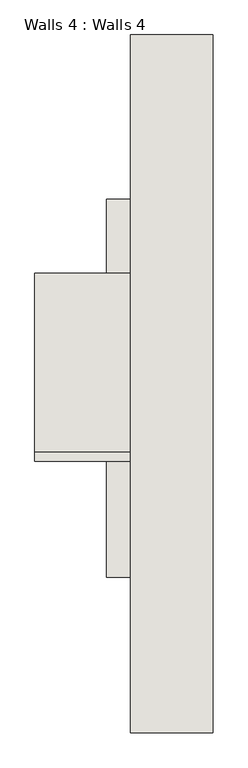
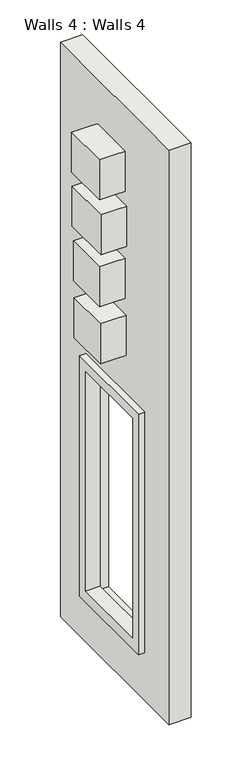
"""IFC4 building model written with IfcOpenShell, lengths in millimetres: wall geometry, Walls 4 : Walls 4."""

from ifc_helpers import new_model, si_unit, frame, origin, place, context, project, spatial, polyline, outline, extrude, source, transform, mapped, element, save


def walls_4_walls_4_b785277b(model_context):
    return source(origin(), model_context, "Body", "SweptSolid", [
        extrude(outline(polyline([(6427.4159582, 6704.0510511), (7343.1184239, 6704.0510511), (7343.1184239, 4418.0510511), (6427.4159582, 4418.0510511), (6427.4159582, 6704.0510511)]), holes=[polyline([(6521.2652695, 6605.6899595), (6521.2652695, 4522.8899595), (7251.0434239, 4522.8899595), (7251.0434239, 6605.6899595), (6521.2652695, 6605.6899595)])]), frame((-12584.6161086, 0.0, 0.0), z_axis=(1.0, 0.0, 0.0), x_axis=(0.0, 1.0, 0.0)), (0.0, 0.0, 1.0), 130.7077729),
        extrude(outline(polyline([(-12758.7083357, 6731.4650508), (-12758.7083357, 7163.2483652), (-12390.4083357, 7163.2483652), (-12390.4083357, 6731.4650508), (-12758.7083357, 6731.4650508)])), frame((0.0, 0.0, 8615.3806189), z_axis=(0.0, 0.0, 1.0), x_axis=(1.0, 0.0, 0.0)), (0.0, 0.0, 1.0), 381.0),
        extrude(outline(polyline([(-12758.7083357, 6708.0602057), (-12758.7083357, 7156.2054395), (-12390.4083357, 7156.2054395), (-12390.4083357, 6708.0602057), (-12758.7083357, 6708.0602057)])), frame((0.0, 0.0, 8107.3806189), z_axis=(0.0, 0.0, 1.0), x_axis=(1.0, 0.0, 0.0)), (0.0, 0.0, 1.0), 381.0),
        extrude(outline(polyline([(-12758.7083357, 6730.7746365), (-12758.7083357, 7137.037243), (-12390.4083357, 7137.037243), (-12390.4083357, 6730.7746365), (-12758.7083357, 6730.7746365)])), frame((0.0, 0.0, 7599.3806189), z_axis=(0.0, 0.0, 1.0), x_axis=(1.0, 0.0, 0.0)), (0.0, 0.0, 1.0), 381.0),
        extrude(outline(polyline([(-12758.7083357, 6716.4341079), (-12758.7083357, 7126.5003631), (-12390.4083357, 7126.5003631), (-12390.4083357, 6716.4341079), (-12758.7083357, 6716.4341079)])), frame((0.0, 0.0, 7065.9806189), z_axis=(0.0, 0.0, 1.0), x_axis=(1.0, 0.0, 0.0)), (0.0, 0.0, 1.0), 381.0),
        extrude(outline(polyline([(6050.8287391, 9420.9325813), (7739.873901, 9420.9325813), (7739.873901, 3962.4), (6050.8287391, 3962.4), (6050.8287391, 9420.9325813)]), holes=[polyline([(6427.4159582, 6704.0510511), (6427.4159582, 4418.0510511), (7341.8159582, 4418.0510511), (7341.8159582, 6704.0510511), (6427.4159582, 6704.0510511)])]), frame((-12527.0272545, 0.0, 0.0), z_axis=(1.0, 0.0, 0.0), x_axis=(0.0, 1.0, 0.0)), (0.0, 0.0, 1.0), 200.1189188),
    ])


if __name__ == "__main__":
    model = new_model("IFC4")
    model_context = context("Model", 3, world=origin())
    ifc_project = project(units=[si_unit("LENGTHUNIT", "METRE", prefix="MILLI")], contexts=[model_context])
    site = spatial("IfcSite", under=ifc_project)
    building = spatial("IfcBuilding", under=site)
    placement = place(None, origin())
    walls_4_walls_4_shape = walls_4_walls_4_b785277b(model_context)
    element("IfcWall", 1, ObjectType="Walls 4 : Walls 4", at=placement, inside=building, context=model_context, shape_type="MappedRepresentation", body=[
        mapped(walls_4_walls_4_shape, transform((0.0, 0.0, 0.0), x_axis=(1.0, 0.0, 0.0), y_axis=(0.0, 1.0, 0.0), z_axis=(0.0, 0.0, 1.0))),
    ])
    save(model, "model.ifc")

# Revit data of these elements
# Element 1 (IfcWall, "Walls 4 : Walls 4")
#   Materials on its faces: "Default Wall"
# Materials
#   "Default Wall": colour RGB 128 128 128, transparency 0
